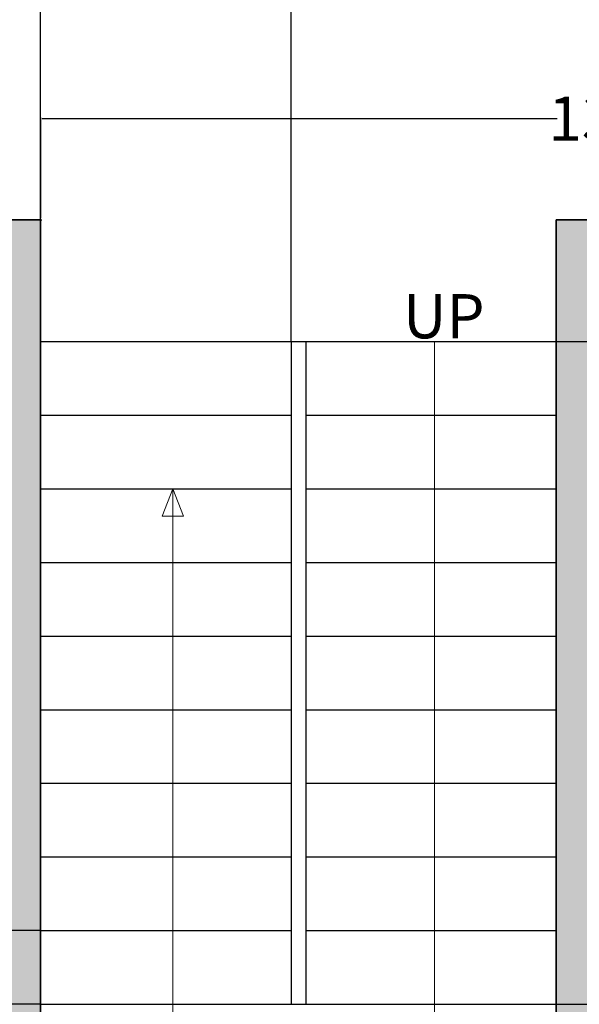
# Model space of a CAD drawing. Units: inches. Extents: x -5 to 482, y -460 to 66.
# Tile 12 of 31: x 142 to 218, y -386 to -252. Entities that reach past the tile are written whole.
import ezdxf

# ---------------------------------------------------------------- set-up
doc = ezdxf.new("R2010")
doc.units = ezdxf.units.IN
doc.header["$MEASUREMENT"] = 0
for name, color, linetype, lineweight in [('A-ANNO-DIMS', 2, 'Continuous', 18), ('A-ANNO-SYMB', 7, 'Continuous', 18), ('A-ANNO-TEXT', 7, 'Continuous', 18), ('A-FLOR-STRS', 7, 'Continuous', 25), ('A-WALL', 7, 'Continuous', 35), ('A-WALL-PATT', 152, 'Continuous', 13)]:
    doc.layers.add(name, color=color, linetype=linetype, lineweight=lineweight)
doc.styles.get("Standard").update_dxf_attribs({"font": 'arial.ttf'})
doc.dimstyles.get("Standard").update_dxf_attribs({"dimtxt": 0.18, "dimasz": 0.18, "dimexe": 0.18, "dimexo": 0.0625, "dimgap": 0.09, "dimtad": 0, "dimtih": 1, "dimtoh": 1, "dimdec": 0, "dimzin": 0, "dimdsep": 46, "dimlunit": 3, "dimtxsty": 'Standard', "dimcen": 0.09, "dimadec": 0, "dimazin": 0, "dimtfac": 1, "dimtdec": 0, "dimtofl": 0, "dimtmove": 0, "dimatfit": 3, "dimfxl": 1, "dimtolj": 1, "dimtzin": 0, "dimarcsym": 0})

# ---------------------------------------------------------------- blocks, each defined once
blk = doc.blocks.new('*D18')
at = {"layer": 'A-ANNO-DIMS', "color": 0, "lineweight": -2, "transparency": 16777216}
for p, q in [((144.44, -144.35), (144.56, -144.35)), ((144.38, -144.53), (144.38, -208.69)), ((144.38, -279.17), (144.38, -215)), ((144.44, -279.35), (144.56, -279.35))]:
    blk.add_line(p, q, dxfattribs=at)
at = {"layer": 'A-ANNO-DIMS', "color": 0, "transparency": 16777216}
for points in [[(144.35, -144.53), (144.41, -144.53), (144.38, -144.35)], [(144.35, -279.17), (144.41, -279.17), (144.38, -279.35)]]:
    blk.add_solid(points, dxfattribs=at)
at = {"layer": 'Defpoints', "color": 0, "transparency": 16777216}
for p in [(144.38, -144.35), (144.38, -144.35), (144.38, -279.35)]:
    blk.add_point(p, dxfattribs=at)
at = {"layer": 'A-ANNO-DIMS', "color": 0, "transparency": 16777216, "insert": (144.38, -211.85), "char_height": 6, "attachment_point": 5}
blk.add_mtext('\\A1;11\'-3"', dxfattribs=at)
blk = doc.blocks.new('*D20')
at = {"layer": 'A-ANNO-DIMS', "color": 0, "lineweight": -2, "transparency": 16777216}
for p, q in [((144.41, -279.11), (144.41, -265.44)), ((144.59, -265.62), (214.53, -265.62)), ((304.7, -265.62), (234.75, -265.62)), ((304.88, -279.11), (304.88, -265.44))]:
    blk.add_line(p, q, dxfattribs=at)
at = {"layer": 'A-ANNO-DIMS', "color": 0, "transparency": 16777216}
for points in [[(144.59, -265.59), (144.59, -265.65), (144.41, -265.62)], [(304.7, -265.59), (304.7, -265.65), (304.88, -265.62)]]:
    blk.add_solid(points, dxfattribs=at)
at = {"layer": 'Defpoints', "color": 0, "transparency": 16777216}
for p in [(304.88, -265.62), (144.41, -279.17), (304.88, -279.17)]:
    blk.add_point(p, dxfattribs=at)
at = {"layer": 'A-ANNO-DIMS', "color": 0, "transparency": 16777216, "insert": (224.64, -265.62), "char_height": 6, "attachment_point": 5}
blk.add_mtext('\\A1;13\'-4"', dxfattribs=at)
blk = doc.blocks.new('*D72')
at = {"layer": 'A-ANNO-DIMS', "color": 0, "lineweight": -2, "transparency": 16777216}
for p, q in [((144.31, -375.86), (-4.9, -375.86)), ((-4.72, -376.04), (-4.72, -380.68)), ((-4.72, -385.68), (-4.72, -381.04)), ((144.31, -385.86), (-4.9, -385.86))]:
    blk.add_line(p, q, dxfattribs=at)
at = {"layer": 'A-ANNO-DIMS', "color": 0, "transparency": 16777216}
for points in [[(-4.75, -376.04), (-4.69, -376.04), (-4.72, -375.86)], [(-4.75, -385.68), (-4.69, -385.68), (-4.72, -385.86)]]:
    blk.add_solid(points, dxfattribs=at)
at = {"layer": 'Defpoints', "color": 0, "transparency": 16777216}
for p in [(144.38, -375.86), (-4.72, -385.86), (144.38, -385.86)]:
    blk.add_point(p, dxfattribs=at)
at = {"layer": 'A-ANNO-DIMS', "color": 0, "transparency": 16777216, "insert": (-4.72, -380.86), "char_height": 0.18, "attachment_point": 5}
blk.add_mtext('\\A1;0\'-10"', dxfattribs=at)
blk = doc.blocks.new('*D73')
at = {"layer": 'A-ANNO-DIMS', "color": 0, "lineweight": -2, "transparency": 16777216}
for p, q in [((144.38, -295.8), (144.38, 50.93)), ((178.38, -295.8), (178.38, 50.93)), ((144.56, 50.75), (160.98, 50.75)), ((178.2, 50.75), (161.78, 50.75))]:
    blk.add_line(p, q, dxfattribs=at)
at = {"layer": 'A-ANNO-DIMS', "color": 0, "transparency": 16777216}
for points in [[(144.56, 50.78), (144.56, 50.72), (144.38, 50.75)], [(178.2, 50.78), (178.2, 50.72), (178.38, 50.75)]]:
    blk.add_solid(points, dxfattribs=at)
at = {"layer": 'Defpoints', "color": 0, "transparency": 16777216}
for p in [(178.38, 50.75), (144.38, -295.86), (178.38, -295.86)]:
    blk.add_point(p, dxfattribs=at)
at = {"layer": 'A-ANNO-DIMS', "color": 0, "transparency": 16777216, "insert": (161.38, 50.75), "char_height": 0.18, "attachment_point": 5}
blk.add_mtext('\\A1;2\'-10"', dxfattribs=at)
blk = doc.blocks.new('*D74')
at = {"layer": 'A-ANNO-DIMS', "color": 0, "lineweight": -2, "transparency": 16777216}
for p, q in [((214.44, -295.86), (468.16, -295.86)), ((467.98, -296.04), (467.98, -340.68)), ((467.98, -385.68), (467.98, -341.04)), ((214.44, -385.86), (468.16, -385.86))]:
    blk.add_line(p, q, dxfattribs=at)
at = {"layer": 'A-ANNO-DIMS', "color": 0, "transparency": 16777216}
for points in [[(467.95, -296.04), (468.01, -296.04), (467.98, -295.86)], [(467.95, -385.68), (468.01, -385.68), (467.98, -385.86)]]:
    blk.add_solid(points, dxfattribs=at)
at = {"layer": 'Defpoints', "color": 0, "transparency": 16777216}
for p in [(214.38, -295.86), (467.98, -295.86), (214.38, -385.86)]:
    blk.add_point(p, dxfattribs=at)
at = {"layer": 'A-ANNO-DIMS', "color": 0, "transparency": 16777216, "insert": (467.98, -340.86), "char_height": 0.18, "attachment_point": 5}
blk.add_mtext('\\A1;7\'-6"', dxfattribs=at)

msp = doc.modelspace()

# ---------------------------------------------------------------- hatches: boundary and pattern name
at = {"layer": 'A-WALL-PATT'}
h = msp.add_hatch(color=256, dxfattribs=at)
h.dxf.hatch_style = 1
h.paths.add_polyline_path([(149.38, -412.85), (144.38, -412.85), (144.38, -283.85), (144.38, -279.35), (133.88, -279.35), (133.88, -283.85), (139.88, -283.85), (139.88, -412.85), (133.51, -412.85), (133.51, -413.92), (102.65, -413.92), (102.65, -421.02), (133.51, -421.02), (133.51, -421.85), (149.38, -421.85)])
h.paths.add_polyline_path([(226.05, -412.85), (218.88, -412.85), (218.88, -350.85), (262.88, -350.85), (262.88, -386.85), (267.38, -386.85), (267.38, -283.85), (270.38, -283.85), (270.38, -279.35), (244.88, -279.35), (244.88, -283.85), (262.88, -283.85), (262.88, -346.35), (218.88, -346.35), (218.88, -283.85), (220.88, -283.85), (220.88, -279.35), (214.38, -279.35), (214.38, -283.85), (214.38, -412.85), (209.38, -412.85), (209.38, -421.85), (226.05, -421.85)])
h.paths.add_polyline_path([(315.81, -412.85), (250.05, -412.85), (250.05, -421.85), (315.81, -421.85)])
h.paths.add_polyline_path([(430.38, -378.35), (421.38, -378.35), (421.38, -412.85), (375.81, -412.85), (375.81, -421.85), (430.38, -421.85)])
h.paths.add_polyline_path([(78.69, -413.92), (47.68, -413.92), (47.68, -412.85), (41.88, -412.85), (41.88, -283.85), (109.88, -283.85), (109.88, -279.35), (41.88, -279.35), (41.88, -241.85), (32.88, -241.85), (32.88, -421.85), (47.68, -421.85), (47.68, -421.02), (78.69, -421.02)])
h.paths.add_polyline_path([(41.88, -144.35), (154.38, -144.35), (154.38, -137.85), (149.88, -137.85), (149.88, -139.85), (41.88, -139.85), (41.88, -97.85), (32.88, -97.85), (32.88, -181.85), (41.88, -181.85)])
h.paths.add_polyline_path([(430.38, -241.85), (421.38, -241.85), (421.38, -279.35), (309.38, -279.35), (309.38, -170.35), (304.88, -170.35), (304.88, -279.35), (294.38, -279.35), (294.38, -283.85), (421.38, -283.85), (421.38, -318.35), (430.38, -318.35)])
h.paths.add_polyline_path([(430.38, -119.85), (421.38, -119.85), (421.38, -139.85), (419.38, -139.85), (419.38, -144.35), (421.38, -144.35), (421.38, -181.85), (430.38, -181.85)])
h.paths.add_polyline_path([(395.38, -139.85), (377.38, -139.85), (377.38, -75.85), (421.38, -75.85), (421.38, -95.85), (430.38, -95.85), (430.38, -45.6), (421.38, -45.6), (421.38, -71.35), (377.38, -71.35), (377.38, -22.85), (372.88, -22.85), (372.88, -139.85), (242.88, -139.85), (242.88, -137.85), (238.38, -137.85), (238.38, -144.35), (304.88, -144.35), (304.88, -146.35), (309.38, -146.35), (309.38, -144.35), (395.38, -144.35)])
h.paths.add_polyline_path([(65.88, 13.15), (32.88, 13.15), (32.88, -37.85), (41.88, -37.85), (41.88, 4.15), (65.88, 4.15)])
h.paths.add_polyline_path([(166.38, 13.15), (125.88, 13.15), (125.88, 4.15), (149.88, 4.15), (149.88, -113.85), (154.38, -113.85), (154.38, 4.15), (166.38, 4.15)])
h.paths.add_polyline_path([(277.88, 13.15), (226.38, 13.15), (226.38, 4.15), (238.38, 4.15), (238.38, -113.85), (242.88, -113.85), (242.88, 4.15), (277.88, 4.15)])
h.paths.add_polyline_path([(430.38, 13.15), (337.88, 13.15), (337.88, 4.15), (372.88, 4.15), (372.88, 1.15), (377.38, 1.15), (377.38, 4.15), (421.38, 4.15), (421.38, -21.6), (430.38, -21.6)])

# ---------------------------------------------------------------- linework, layer by layer
at = {"layer": 'A-ANNO-SYMB'}
for p, q in [((197.88, -295.86), (197.88, -395.39)), ((162.32, -315.86), (160.86, -319.59)), ((162.32, -395.39), (162.32, -315.86)), ((162.32, -315.86), (163.78, -319.59)), ((160.86, -319.59), (162.32, -319.59)), ((163.78, -319.59), (162.32, -319.59))]:
    msp.add_line(p, q, dxfattribs=at)
at = {"layer": 'A-FLOR-STRS'}
for p, q in [((144.38, -295.86), (214.38, -295.86)), ((178.38, -295.86), (178.38, -385.86)), ((180.38, -295.86), (180.38, -385.86)), ((144.38, -305.86), (178.38, -305.86)), ((180.38, -305.86), (214.38, -305.86)), ((144.38, -315.86), (178.38, -315.86)), ((180.38, -315.86), (214.38, -315.86)), ((144.38, -325.86), (178.38, -325.86)), ((180.38, -325.86), (214.38, -325.86)), ((144.38, -335.86), (178.38, -335.86)), ((180.38, -335.86), (214.38, -335.86)), ((144.38, -345.86), (178.38, -345.86)), ((180.38, -345.86), (214.38, -345.86)), ((144.38, -355.86), (178.38, -355.86)), ((180.38, -355.86), (214.38, -355.86)), ((144.38, -365.86), (178.38, -365.86)), ((180.38, -365.86), (214.38, -365.86)), ((144.38, -375.86), (178.38, -375.86)), ((180.38, -375.86), (214.38, -375.86)), ((144.38, -385.86), (214.38, -385.86))]:
    msp.add_line(p, q, dxfattribs=at)
at = {"layer": 'A-WALL'}
for p, q in [((133.88, -279.35), (144.38, -279.35)), ((144.38, -283.85), (144.38, -279.35)), ((214.38, -283.85), (214.38, -279.35)), ((214.38, -279.35), (220.88, -279.35)), ((144.38, -283.85), (144.38, -412.85)), ((214.38, -283.85), (214.38, -412.85))]:
    msp.add_line(p, q, dxfattribs=at)

# ---------------------------------------------------------------- texts
at = {"layer": 'A-ANNO-TEXT', "insert": (193.58, -289.44), "char_height": 6, "attachment_point": 1}
msp.add_mtext('UP', dxfattribs=at)

# ---------------------------------------------------------------- dimensions: what is measured, and where the dimension line sits
at = {"layer": 'A-ANNO-DIMS'}
for base, p1, p2, override, picture, middle in [((178.38, 50.75), (144.38, -295.86), (178.38, -295.86), {"dimdec": 1, "dimlfac": 1, "dimrnd": 0, "dimzin": 1, "dimdsep": 46, "dimlunit": 4, "dimfrac": 2}, '*D73', (161.38, 50.75)), ((304.88, -265.62), (144.41, -279.17), (304.88, -279.17), {"dimtxt": 6, "dimclrd": 0, "dimclre": 0, "dimclrt": 0}, '*D20', (224.64, -265.62))]:
    dim = msp.add_linear_dim(base=base, p1=p1, p2=p2, dimstyle='Standard', override=override, dxfattribs=at)
    dim.commit()
    dim.dimension.update_dxf_attribs({"geometry": picture, "text_midpoint": middle})
for base, p1, p2, override, picture, middle in [((144.38, -144.35), (144.38, -279.35), (144.38, -144.35), {"dimtxt": 6, "dimclrd": 0, "dimclre": 0, "dimclrt": 0}, '*D18', (144.38, -211.85)), ((467.98, -295.86), (214.38, -385.86), (214.38, -295.86), {"dimdec": 1, "dimlfac": 1, "dimrnd": 0, "dimzin": 1, "dimdsep": 46, "dimlunit": 4, "dimfrac": 2}, '*D74', (467.98, -340.86)), ((-4.72, -385.86), (144.38, -375.86), (144.38, -385.86), {"dimdec": 1, "dimlfac": 1, "dimrnd": 0, "dimzin": 1, "dimdsep": 46, "dimlunit": 4, "dimfrac": 2}, '*D72', (-4.72, -380.86))]:
    dim = msp.add_linear_dim(base=base, p1=p1, p2=p2, angle=90, dimstyle='Standard', override=override, dxfattribs=at)
    dim.commit()
    dim.dimension.update_dxf_attribs({"geometry": picture, "text_midpoint": middle})

doc.saveas('drawing.dxf')
